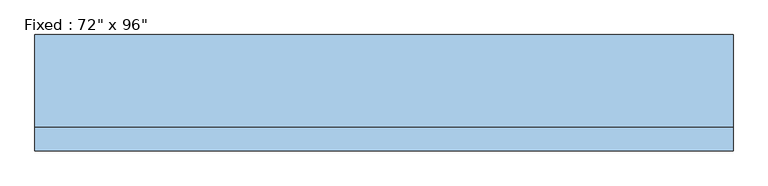
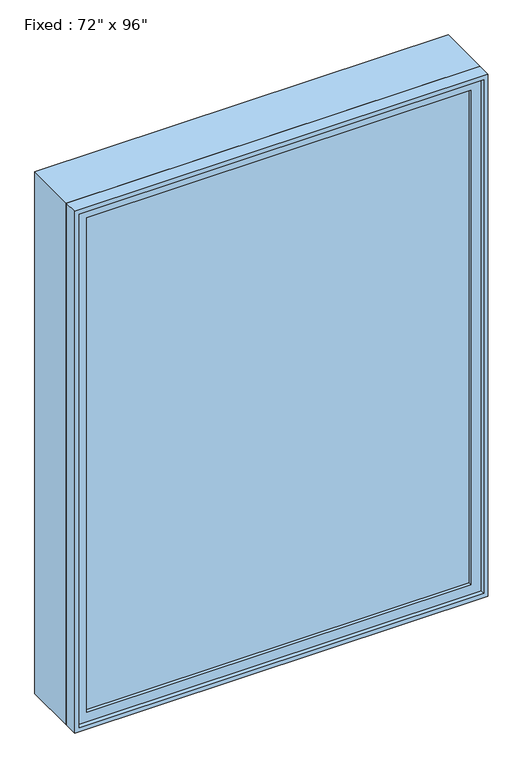
"""IFC4 building model written with IfcOpenShell, lengths in millimetres: window geometry."""

from ifc_helpers import new_model, si_unit, frame, origin, place, context, project, spatial, polyline, outline, extrude, source, transform, mapped, element, save


def window_9610881e(model_context):
    return source(origin(), model_context, "Body", "SweptSolid", [
        extrude(outline(polyline([(812.8, -104.775), (812.8, -117.475), (-889.0, -117.475), (-889.0, -104.775), (812.8, -104.775)])), frame((0.0, 0.0, 368.3), z_axis=(0.0, 0.0, 1.0), x_axis=(1.0, 0.0, 0.0)), (0.0, 0.0, 1.0), 2311.4),
        extrude(outline(polyline([(2724.15, -933.45), (323.85, -933.45), (323.85, 857.25), (2724.15, 857.25), (2724.15, -933.45)]), holes=[polyline([(2679.7, -889.0), (2679.7, 812.8), (368.3, 812.8), (368.3, -889.0), (2679.7, -889.0)])]), frame((0.0, -133.35, 0.0), z_axis=(0.0, 1.0, 0.0), x_axis=(0.0, 0.0, 1.0)), (0.0, 0.0, 1.0), 44.45),
        extrude(outline(polyline([(2743.2, -952.5), (304.8, -952.5), (304.8, 876.3), (2743.2, 876.3), (2743.2, -952.5)]), holes=[polyline([(2711.45, -920.75), (2711.45, 844.55), (336.55, 844.55), (336.55, -920.75), (2711.45, -920.75)])]), frame((0.0, -88.9, 0.0), z_axis=(0.0, 1.0, 0.0), x_axis=(0.0, 0.0, 1.0)), (0.0, 0.0, 1.0), 241.3),
        extrude(outline(polyline([(2743.2, 876.3), (2743.2, -952.5), (304.8, -952.5), (304.8, 876.3), (2743.2, 876.3)]), holes=[polyline([(2724.15, 857.25), (323.85, 857.25), (323.85, -933.45), (2724.15, -933.45), (2724.15, 857.25)])]), frame((0.0, -152.4, 0.0), z_axis=(0.0, 1.0, 0.0), x_axis=(0.0, 0.0, 1.0)), (0.0, 0.0, 1.0), 63.5),
    ])


if __name__ == "__main__":
    model = new_model("IFC4")
    model_context = context("Model", 3, world=origin())
    ifc_project = project(units=[si_unit("LENGTHUNIT", "METRE", prefix="MILLI")], contexts=[model_context])
    site = spatial("IfcSite", under=ifc_project)
    building = spatial("IfcBuilding", under=site)
    placement = place(None, origin())
    window_shape = window_9610881e(model_context)
    element("IfcWindow", 1, ObjectType="Fixed : 72\" x 96\"", at=placement, inside=building, context=model_context, shape_type="MappedRepresentation", body=[
        mapped(window_shape, transform((0.0, 0.0, 0.0), x_axis=(1.0, 0.0, 0.0), y_axis=(0.0, 1.0, 0.0), z_axis=(0.0, 0.0, 1.0))),
    ])
    save(model, "model.ifc")

# Revit data of these elements
# Type "Fixed : 72\" x 96\""
#   Type Mark = "11"
#   Construction Type Id = "GSP4R"
#   Assembly Code = "B2020100"
#   Analytic Construction = "1/8 in Pilkington single glazing"
#   Visual Light Transmittance = 0.9
#   Solar Heat Gain Coefficient = 0.78
#   Heat Transfer Coefficient (U) = 0.6496 BTU/(h·ft²·°F)
#   Height = 8' - 0"
#   Default Sill Height = 1' - 0"
#   Width = 6' - 0"
#   Window Inset = 0' - 0 3/4"
#   Define Thermal Properties by = 1
#   Glass Pane Material = Glass
#   Sash Material = Iron, Ductile
#   Wall Closure = (empty or 0)
# Element 1 (IfcWindow, "Fixed : 72\" x 96\"")
#   Materials on its faces: "Iron, Ductile", "Glass"
# Materials
#   "Glass": class "Glass", colour RGB 0 128 192, transparency 0.75, Description = "Soda Lime Glass", Cost = 0
#   "Iron, Ductile": class "Metal", colour RGB 0 0 0, transparency 0, Description = "Ductile cast iron", Cost = 0
